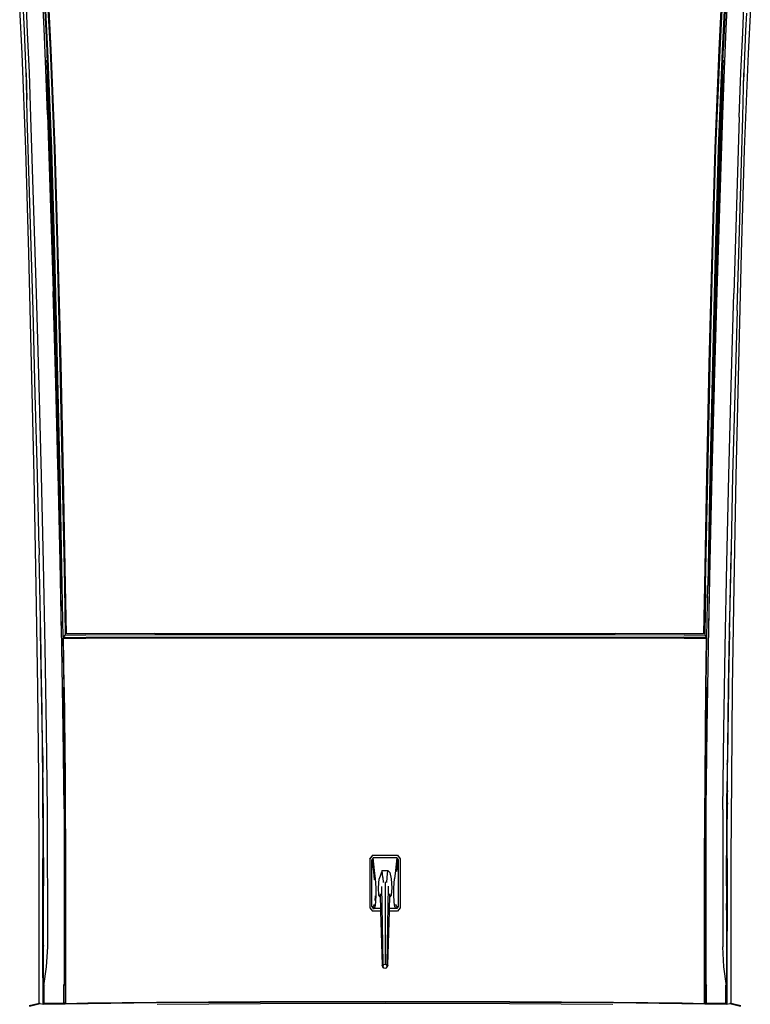
# Model space of a CAD drawing. Units: inches. Extents: x -4737294 to -4736756, y 1716389 to 1717040.
# Tile 9 of 25: x -4737175 to -4737124, y 1716491 to 1716559. Entities that reach past the tile are written whole.
import ezdxf

# ---------------------------------------------------------------- set-up
doc = ezdxf.new("R2010")
doc.units = ezdxf.units.IN
doc.header["$MEASUREMENT"] = 0
doc.layers.add('A-EQPM-VEHI', color=250, linetype='Continuous', lineweight=13)
doc.layers.add('Edges', color=250, linetype='Continuous')

# ---------------------------------------------------------------- blocks, each defined once
blk = doc.blocks.new('Nissan Qashqai pl')
at = {"layer": 'Edges'}
for p, q in [((9.4782, 12.5024), (9.5503, 12.4987)), ((9.5168, 12.4903), (9.4761, 12.4919)), ((9.4862, 12.4961), (9.514, 12.4949)), ((9.514, 12.4949), (9.5811, 12.492)), ((9.5812, 12.4874), (9.5168, 12.4903)), ((9.5503, 12.4987), (9.7029, 12.4926)), ((9.651, 12.4906), (9.5811, 12.492)), ((9.5811, 12.492), (9.594, 12.4914)), ((9.6514, 12.4849), (9.5812, 12.4874)), ((9.9583, 12.4812), (9.651, 12.4906)), ((9.7029, 12.4926), (9.8673, 12.4878)), ((9.8673, 12.4878), (10.0423, 12.4835)), ((11.0581, 12.4738), (11.0614, 12.4872)), ((11.0582, 12.47), (11.0624, 12.4866)), ((9.6514, 12.4849), (9.9312, 12.4761)), ((10.0776, 12.4719), (9.9312, 12.4761)), ((9.9583, 12.4812), (10.091, 12.4775)), ((10.0423, 12.4835), (10.2211, 12.4795)), ((10.2201, 12.4683), (10.0776, 12.4719)), ((10.091, 12.4775), (10.2202, 12.4743)), ((10.2202, 12.4743), (10.2203, 12.4743)), ((10.2203, 12.4743), (10.3353, 12.4717)), ((10.2211, 12.4795), (10.3955, 12.4762)), ((10.3353, 12.4717), (10.4477, 12.4694)), ((10.3353, 12.4717), (10.346, 12.4714)), ((10.346, 12.4714), (10.4477, 12.4694)), ((10.3955, 12.4762), (10.5572, 12.4737)), ((10.5572, 12.4737), (10.7004, 12.4722)), ((10.7004, 12.4722), (10.8279, 12.4715)), ((10.8279, 12.4715), (11.0544, 12.4714)), ((11.0544, 12.4714), (11.0575, 12.4714)), ((11.0575, 12.4714), (11.0581, 12.4738)), ((11.0575, 12.4714), (11.0582, 12.47)), ((11.0592, 12.4653), (11.0582, 12.47)), ((9.4694, 12.4654), (9.5105, 12.4637)), ((9.4706, 12.4561), (9.5443, 12.4522)), ((9.5446, 12.4542), (9.4709, 12.4581)), ((9.472, 12.463), (9.5454, 12.4591)), ((9.472, 12.4614), (9.5454, 12.4576)), ((9.5105, 12.4637), (9.5755, 12.4608)), ((9.5454, 12.4591), (9.5454, 12.4593)), ((9.5695, 12.4589), (9.5454, 12.4591)), ((9.5454, 12.4576), (9.7014, 12.4513)), ((9.5609, 12.4593), (9.5695, 12.4589)), ((9.5786, 12.4588), (9.5695, 12.4589)), ((9.5695, 12.4589), (9.7014, 12.4536)), ((9.5755, 12.4608), (9.6472, 12.4581)), ((9.6206, 12.4581), (9.5786, 12.4588)), ((9.6714, 12.4567), (9.6206, 12.4581)), ((9.6414, 12.458), (9.6407, 12.458)), ((9.6472, 12.4581), (9.9278, 12.4492)), ((9.6549, 12.4576), (9.6558, 12.4574)), ((9.6825, 12.4564), (9.6714, 12.4567)), ((9.6825, 12.4564), (9.6829, 12.4563)), ((9.6943, 12.456), (9.6825, 12.4564)), ((9.6943, 12.4558), (9.6943, 12.456)), ((9.6951, 12.456), (9.6943, 12.456)), ((9.6951, 12.4558), (9.6951, 12.456)), ((9.8565, 12.451), (9.6951, 12.456)), ((10.3586, 12.4651), (10.2201, 12.4683)), ((10.4931, 12.4624), (10.3586, 12.4651)), ((10.4477, 12.4694), (10.4538, 12.4693)), ((10.4538, 12.4693), (10.4681, 12.469)), ((10.4676, 12.4691), (10.4538, 12.4693)), ((10.5566, 12.4677), (10.4676, 12.4691)), ((10.4676, 12.4691), (10.546, 12.4677)), ((10.4681, 12.469), (10.5866, 12.467)), ((10.6237, 12.4603), (10.4931, 12.4624)), ((10.546, 12.4677), (10.546, 12.4678)), ((10.546, 12.4677), (10.5576, 12.4675)), ((10.7, 12.4662), (10.5566, 12.4677)), ((10.5576, 12.4675), (10.6649, 12.4659)), ((10.5866, 12.467), (10.6649, 12.4659)), ((10.7502, 12.4586), (10.6237, 12.4603)), ((10.6649, 12.4659), (10.6786, 12.4658)), ((10.6649, 12.4659), (10.6772, 12.4657)), ((10.6786, 12.4657), (10.6772, 12.4657)), ((10.6786, 12.4658), (10.6786, 12.4662)), ((10.6786, 12.4657), (10.6786, 12.4658)), ((10.6786, 12.4658), (10.6801, 12.4657)), ((10.6786, 12.4657), (10.6801, 12.4657)), ((10.6801, 12.4662), (10.6801, 12.4657)), ((10.6801, 12.4657), (10.6801, 12.4657)), ((10.6801, 12.4657), (10.6811, 12.4657)), ((10.6801, 12.4657), (10.6811, 12.4657)), ((10.6811, 12.4662), (10.6811, 12.4657)), ((10.6811, 12.4657), (10.6811, 12.4657)), ((10.6811, 12.4657), (10.6966, 12.4654)), ((10.6811, 12.4657), (10.6991, 12.4655)), ((10.6811, 12.4657), (10.6991, 12.4655)), ((10.6966, 12.4654), (10.7144, 12.4653)), ((10.6991, 12.4655), (10.7144, 12.4653)), ((10.7201, 12.4661), (10.7, 12.4662)), ((10.7144, 12.4653), (10.7239, 12.4653)), ((10.7201, 12.4661), (10.7306, 12.4653)), ((10.7395, 12.4659), (10.7201, 12.4661)), ((10.7239, 12.4653), (10.7248, 12.4653)), ((10.7306, 12.4653), (10.7248, 12.4653)), ((10.7311, 12.4652), (10.7306, 12.4653)), ((10.7495, 12.4652), (10.7311, 12.4652)), ((10.7311, 12.4652), (10.7502, 12.4651)), ((10.7395, 12.4659), (10.7495, 12.4652)), ((10.7923, 12.4656), (10.7395, 12.4659)), ((10.8179, 12.4648), (10.7495, 12.4652)), ((10.7502, 12.4651), (10.7504, 12.4651)), ((10.7502, 12.4586), (10.968, 12.4585)), ((10.7504, 12.4651), (10.7808, 12.4649)), ((10.7808, 12.4649), (10.8179, 12.4648)), ((10.7923, 12.4652), (10.7923, 12.4656)), ((10.7933, 12.4656), (10.7923, 12.4656)), ((10.7933, 12.4652), (10.7933, 12.4656)), ((10.804, 12.4656), (10.7933, 12.4656)), ((10.804, 12.4653), (10.804, 12.4656)), ((10.8075, 12.4655), (10.804, 12.4656)), ((10.8075, 12.4655), (10.8075, 12.4653)), ((10.811, 12.4655), (10.8075, 12.4655)), ((10.811, 12.4655), (10.811, 12.4653)), ((10.8145, 12.4655), (10.811, 12.4655)), ((10.8145, 12.4653), (10.8145, 12.4655)), ((10.8279, 12.4654), (10.8145, 12.4655)), ((10.8277, 12.4647), (10.8179, 12.4648)), ((10.8711, 12.4646), (10.8277, 12.4647)), ((10.8279, 12.4654), (11.0592, 12.4653)), ((10.8711, 12.4646), (10.8824, 12.4646)), ((10.8824, 12.4646), (10.8825, 12.4646)), ((10.8825, 12.4646), (10.8884, 12.4646)), ((10.8884, 12.4646), (10.8923, 12.4646)), ((10.8923, 12.4646), (10.8996, 12.4646)), ((10.9097, 12.4646), (10.8996, 12.4646)), ((10.9097, 12.4646), (10.9399, 12.4646)), ((10.9399, 12.4646), (10.9491, 12.4645)), ((10.9491, 12.4645), (11.0301, 12.4645)), ((11, 12.4605), (10.968, 12.4585)), ((11.0301, 12.4645), (11, 12.4605)), ((11.0301, 12.4637), (11.0287, 12.4637)), ((11.03, 12.4635), (11.0301, 12.4637)), ((11.0301, 12.4642), (11.0301, 12.4645)), ((11.0574, 12.4637), (11.0301, 12.4637)), ((11.0568, 12.4323), (11.0574, 12.4637)), ((11.0574, 12.4637), (11.0592, 12.4653)), ((11.0585, 12.43), (11.0592, 12.4653)), ((9.5443, 12.4522), (9.701, 12.4459)), ((9.7011, 12.4478), (9.5446, 12.4542)), ((9.701, 12.4459), (9.8673, 12.441)), ((9.8673, 12.443), (9.7011, 12.4478)), ((9.7014, 12.4536), (9.8673, 12.4488)), ((9.7014, 12.4513), (9.8673, 12.4464)), ((9.9794, 12.4475), (9.8565, 12.451)), ((9.8673, 12.4488), (10.0429, 12.4444)), ((9.8673, 12.4464), (10.0429, 12.4421)), ((10.043, 12.4387), (9.8673, 12.443)), ((9.8673, 12.441), (10.0431, 12.4367)), ((9.9278, 12.4492), (10.0747, 12.445)), ((10.0998, 12.4443), (9.9794, 12.4475)), ((10.0429, 12.4444), (10.2216, 12.4404)), ((10.0429, 12.4421), (10.2215, 12.4381)), ((10.2218, 12.4347), (10.043, 12.4387)), ((10.0747, 12.445), (10.078, 12.4449)), ((10.078, 12.4449), (10.2146, 12.4414)), ((10.2146, 12.4414), (10.0998, 12.4443)), ((10.2146, 12.4414), (10.2175, 12.4413)), ((10.2175, 12.4413), (10.3564, 12.4382)), ((10.2216, 12.4404), (10.3947, 12.4371)), ((10.0431, 12.4367), (10.2218, 12.4327)), ((10.2215, 12.4381), (10.3945, 12.4348)), ((10.3947, 12.4314), (10.2218, 12.4347)), ((10.2218, 12.4327), (10.3947, 12.4294)), ((10.3564, 12.4382), (10.4638, 12.436)), ((10.4773, 12.4335), (10.3945, 12.4348)), ((10.3947, 12.4371), (10.4638, 12.436)), ((10.3947, 12.4314), (10.4735, 12.4301)), ((10.3947, 12.4294), (10.4715, 12.4282)), ((10.4638, 12.436), (10.4914, 12.4355)), ((10.4715, 12.4282), (10.4711, 12.3973)), ((10.4731, 12.3973), (10.4735, 12.4301)), ((10.4735, 12.4301), (10.4773, 12.4335)), ((10.4773, 12.4296), (10.4769, 12.3968)), ((10.4773, 12.4335), (10.4773, 12.4296)), ((10.4785, 12.433), (10.4773, 12.4335)), ((10.5561, 12.4323), (10.4773, 12.4335)), ((10.4781, 12.3972), (10.4785, 12.433)), ((10.5563, 12.4318), (10.4785, 12.433)), ((10.4914, 12.4355), (10.6223, 12.4333)), ((10.5561, 12.4323), (10.6996, 12.4308)), ((10.6999, 12.4304), (10.5563, 12.4318)), ((10.6223, 12.4333), (10.7493, 12.4316)), ((10.6996, 12.4308), (10.7722, 12.4304)), ((10.827, 12.4297), (10.6999, 12.4304)), ((10.7493, 12.4316), (11.0294, 12.4315)), ((10.7722, 12.4304), (10.7722, 12.4302)), ((10.7722, 12.4304), (10.7889, 12.4303)), ((10.7889, 12.4302), (10.7889, 12.4303)), ((10.7889, 12.4303), (10.7923, 12.4303)), ((10.7923, 12.4302), (10.7923, 12.4303)), ((10.7923, 12.4303), (10.7933, 12.4303)), ((10.7933, 12.4302), (10.7933, 12.4303)), ((10.7933, 12.4303), (10.8267, 12.4301)), ((10.8267, 12.4301), (11.0585, 12.43)), ((10.9133, 12.4296), (10.827, 12.4297)), ((10.9133, 12.4296), (10.9133, 12.4298)), ((10.9137, 12.4296), (10.9133, 12.4296)), ((10.9137, 12.4296), (10.9138, 12.4298)), ((10.9715, 12.4296), (10.9137, 12.4296)), ((10.9715, 12.4299), (10.9715, 12.4296)), ((11.0579, 12.4296), (10.9715, 12.4296)), ((11.0281, 12.4323), (11.0568, 12.4323)), ((11.0294, 12.4315), (11.0294, 12.4316)), ((11.0295, 12.4341), (11.0295, 12.4343)), ((11.0568, 12.4323), (11.0585, 12.43)), ((11.0572, 12.3942), (11.0579, 12.4296)), ((11.0579, 12.3938), (11.0585, 12.43)), ((11.0579, 12.4296), (11.0585, 12.43)), ((10.4711, 12.3973), (10.4706, 12.2875)), ((10.4726, 12.2875), (10.4731, 12.3973)), ((10.4764, 12.2872), (10.4769, 12.3968)), ((10.4776, 12.2874), (10.4781, 12.3972)), ((11.056, 12.2851), (11.0572, 12.3942)), ((11.0566, 12.2849), (11.0579, 12.3938)), ((10.4706, 11.5566), (10.4706, 12.2875)), ((10.4726, 11.5567), (10.4726, 12.2875)), ((10.4764, 11.5569), (10.4764, 12.2872)), ((10.4776, 11.5567), (10.4776, 12.2874)), ((11.0551, 12.1203), (11.056, 12.2851)), ((11.0557, 12.1202), (11.0566, 12.2849)), ((11.0595, 12.2842), (11.0586, 12.1198)), ((11.0547, 11.9221), (11.0551, 12.1203)), ((11.0554, 11.9221), (11.0557, 12.1202)), ((11.0586, 12.1198), (11.0583, 11.9221)), ((10.8228, 11.9421), (10.8224, 11.9421)), ((10.8228, 11.9421), (10.8283, 11.9461)), ((10.8228, 11.9021), (10.8228, 11.9421)), ((10.827, 11.9408), (10.8301, 11.9431)), ((10.827, 11.9408), (10.827, 11.9033)), ((10.827, 11.9408), (10.8467, 11.9386)), ((10.8279, 11.9461), (10.8283, 11.9461)), ((10.8283, 11.9461), (10.906, 11.9461)), ((10.8483, 11.9406), (10.8301, 11.9431)), ((10.8301, 11.9431), (10.9043, 11.9431)), ((10.8467, 11.9386), (10.8603, 11.9373)), ((10.9035, 11.9403), (10.9008, 11.9391)), ((10.905, 11.9414), (10.9035, 11.9403)), ((10.9043, 11.9431), (10.9074, 11.9408)), ((10.9043, 11.9431), (10.905, 11.9414)), ((10.9074, 11.9393), (10.9057, 11.9384)), ((10.906, 11.9461), (10.9116, 11.9421)), ((10.9074, 11.9408), (10.9074, 11.9393)), ((10.9074, 11.9393), (10.9074, 11.9291)), ((10.9116, 11.9421), (10.9116, 11.929)), ((10.8467, 11.9263), (10.8501, 11.9295)), ((10.8467, 11.9178), (10.8467, 11.9263)), ((10.8579, 11.9255), (10.8467, 11.9263)), ((10.8501, 11.9295), (10.8603, 11.9316)), ((10.8662, 11.925), (10.8579, 11.9255)), ((10.8746, 11.9363), (10.8603, 11.9373)), ((10.8603, 11.9316), (10.8746, 11.9327)), ((10.9946, 11.9254), (10.872, 11.9276)), ((10.8861, 11.9361), (10.8746, 11.9363)), ((10.8746, 11.9327), (10.8861, 11.9319)), ((10.889, 11.9296), (10.884, 11.9298)), ((10.8959, 11.9365), (10.8861, 11.9361)), ((10.8861, 11.9319), (10.889, 11.9296)), ((10.9074, 11.9291), (10.889, 11.9296)), ((10.9021, 11.9372), (10.8959, 11.9365)), ((10.9057, 11.9384), (10.9021, 11.9372)), ((10.9116, 11.929), (10.9074, 11.9291)), ((10.9973, 11.9268), (10.9116, 11.929)), ((10.9969, 11.9247), (10.9946, 11.9254)), ((10.9969, 11.9247), (10.996, 11.9221)), ((10.999, 11.9258), (10.9969, 11.9247)), ((10.9973, 11.9268), (11.0001, 11.9254)), ((10.999, 11.9258), (10.9973, 11.9268)), ((11.0012, 11.9247), (10.999, 11.9258)), ((11.0012, 11.9247), (11.0001, 11.9254)), ((11.002, 11.9221), (11.0012, 11.9247)), ((10.8579, 11.9187), (10.8467, 11.9178)), ((10.8467, 11.9178), (10.8603, 11.9126)), ((10.8579, 11.9187), (10.8662, 11.9191)), ((10.8746, 11.9115), (10.8603, 11.9126)), ((10.8746, 11.9078), (10.8603, 11.9068)), ((10.8647, 11.9221), (10.996, 11.9221)), ((10.8723, 11.9165), (10.9946, 11.9187)), ((10.8861, 11.9122), (10.8746, 11.9115)), ((10.8861, 11.908), (10.8746, 11.9078)), ((10.884, 11.9144), (10.889, 11.9145)), ((10.889, 11.9145), (10.8861, 11.9122)), ((10.8959, 11.9077), (10.8861, 11.908)), ((10.889, 11.9145), (10.9074, 11.915)), ((10.9021, 11.9069), (10.8959, 11.9077)), ((10.9074, 11.915), (10.9116, 11.9151)), ((10.9074, 11.915), (10.9074, 11.9049)), ((10.9116, 11.9151), (10.9973, 11.9173)), ((10.9116, 11.9151), (10.9116, 11.9021)), ((10.9946, 11.9187), (10.9969, 11.9195)), ((10.996, 11.9221), (10.9969, 11.9195)), ((10.9969, 11.9195), (10.999, 11.9184)), ((11.0001, 11.9187), (10.9973, 11.9173)), ((10.9973, 11.9173), (10.999, 11.9184)), ((10.999, 11.9184), (10.9996, 11.9187)), ((10.9996, 11.9187), (11.0012, 11.9195)), ((11.0001, 11.9187), (10.9996, 11.9187)), ((11.0012, 11.9195), (11.0001, 11.9187)), ((11.0012, 11.9195), (11.002, 11.9221)), ((11.0551, 11.7239), (11.0547, 11.9221)), ((11.0557, 11.724), (11.0554, 11.9221)), ((11.0583, 11.9221), (11.0586, 11.7244)), ((10.8224, 11.9021), (10.8228, 11.9021)), ((10.8228, 11.9021), (10.8283, 11.8981)), ((10.8467, 11.9056), (10.827, 11.9033)), ((10.827, 11.9033), (10.8301, 11.9011)), ((10.8283, 11.8981), (10.8279, 11.8981)), ((10.8283, 11.8981), (10.906, 11.8981)), ((10.8301, 11.9011), (10.8483, 11.9036)), ((10.9043, 11.9011), (10.8301, 11.9011)), ((10.8603, 11.9068), (10.8467, 11.9056)), ((10.8483, 11.9036), (10.8619, 11.905)), ((10.8871, 11.9063), (10.8944, 11.906)), ((10.9008, 11.905), (10.9035, 11.9039)), ((10.9057, 11.9058), (10.9021, 11.9069)), ((10.9035, 11.9039), (10.905, 11.9028)), ((10.9043, 11.9011), (10.9074, 11.9033)), ((10.905, 11.9028), (10.9043, 11.9011)), ((10.9074, 11.9049), (10.9057, 11.9058)), ((10.906, 11.8981), (10.9116, 11.9021)), ((10.9074, 11.9033), (10.9074, 11.9049)), ((10.9074, 11.9033), (10.9074, 11.9048)), ((11.056, 11.559), (11.0551, 11.7239)), ((11.0566, 11.5593), (11.0557, 11.724)), ((11.0586, 11.7244), (11.0595, 11.5599)), ((10.4706, 11.5566), (10.4711, 11.4469)), ((10.4731, 11.4469), (10.4726, 11.5567)), ((10.4769, 11.4474), (10.4764, 11.5569)), ((10.4781, 11.4469), (10.4776, 11.5567)), ((11.0572, 11.4499), (11.056, 11.559)), ((11.0579, 11.4504), (11.0566, 11.5593)), ((10.4711, 11.4469), (10.4715, 11.416)), ((10.4735, 11.414), (10.4731, 11.4469)), ((10.4773, 11.4146), (10.4769, 11.4474)), ((10.4785, 11.4111), (10.4781, 11.4469)), ((11.0579, 11.4146), (11.0572, 11.4499)), ((11.0585, 11.4142), (11.0579, 11.4504)), ((10.0431, 11.4075), (9.8673, 11.4031)), ((10.043, 11.4055), (10.2218, 11.4094)), ((10.2218, 11.4114), (10.0431, 11.4075)), ((10.3945, 11.4094), (10.2215, 11.406)), ((10.3947, 11.4148), (10.2218, 11.4114)), ((10.2218, 11.4094), (10.3947, 11.4128)), ((10.4416, 11.4077), (10.3564, 11.406)), ((10.4773, 11.4107), (10.3945, 11.4094)), ((10.4715, 11.416), (10.3947, 11.4148)), ((10.3947, 11.4128), (10.4735, 11.414)), ((10.4416, 11.4078), (10.3947, 11.4071)), ((10.4519, 11.4079), (10.4416, 11.4077)), ((10.4519, 11.4079), (10.4416, 11.4078)), ((10.4416, 11.4077), (10.4416, 11.4078)), ((10.4524, 11.408), (10.4519, 11.4079)), ((10.4519, 11.4079), (10.4519, 11.4079)), ((10.4524, 11.4079), (10.4519, 11.4079)), ((10.4524, 11.4079), (10.4524, 11.408)), ((10.4533, 11.408), (10.4524, 11.408)), ((10.4533, 11.4079), (10.4524, 11.4079)), ((10.4638, 11.4081), (10.4533, 11.4079)), ((10.4638, 11.4081), (10.4533, 11.408)), ((10.4533, 11.4079), (10.4533, 11.408)), ((10.4914, 11.4087), (10.4638, 11.4081)), ((10.4773, 11.4107), (10.4735, 11.414)), ((10.4773, 11.4146), (10.4773, 11.4107)), ((10.4773, 11.4107), (10.5561, 11.4119)), ((10.4773, 11.4107), (10.4785, 11.4111)), ((10.5563, 11.4123), (10.4785, 11.4111)), ((10.6223, 11.4109), (10.4914, 11.4087)), ((10.6996, 11.4134), (10.5561, 11.4119)), ((10.5563, 11.4123), (10.6999, 11.4138)), ((10.7493, 11.4125), (10.6223, 11.4109)), ((10.7722, 11.4138), (10.6996, 11.4134)), ((10.6999, 11.4138), (10.7722, 11.4142)), ((10.7493, 11.4125), (11.0294, 11.4126)), ((10.7722, 11.4142), (10.7889, 11.4143)), ((10.7722, 11.4142), (10.7722, 11.4138)), ((10.7889, 11.4139), (10.7722, 11.4138)), ((10.7889, 11.4139), (10.7889, 11.4143)), ((10.7889, 11.4143), (10.7923, 11.4143)), ((10.7923, 11.4139), (10.7889, 11.4139)), ((10.7923, 11.4139), (10.7923, 11.4143)), ((10.7923, 11.4143), (10.7933, 11.4143)), ((10.7933, 11.4139), (10.7923, 11.4139)), ((10.7933, 11.4143), (10.827, 11.4145)), ((10.7933, 11.4139), (10.7933, 11.4143)), ((10.8267, 11.4141), (10.7933, 11.4139)), ((10.8267, 11.4141), (11.0585, 11.4142)), ((10.827, 11.4145), (11.0579, 11.4146)), ((11.0294, 11.4118), (11.0281, 11.4118)), ((11.0294, 11.4125), (11.0294, 11.4126)), ((11.0295, 11.4116), (11.0294, 11.4118)), ((11.0568, 11.4118), (11.0294, 11.4118)), ((11.0585, 11.4142), (11.0568, 11.4118)), ((11.0574, 11.3804), (11.0568, 11.4118)), ((11.0585, 11.4142), (11.0579, 11.4146)), ((11.0592, 11.3789), (11.0585, 11.4142)), ((9.5443, 11.3919), (9.4706, 11.388)), ((9.701, 11.3983), (9.5443, 11.3919)), ((9.5446, 11.39), (9.7011, 11.3963)), ((9.7014, 11.3929), (9.5454, 11.3866)), ((9.6472, 11.3861), (9.9278, 11.3949)), ((9.6714, 11.3874), (9.8565, 11.3931)), ((9.8673, 11.4031), (9.701, 11.3983)), ((9.7011, 11.3963), (9.8673, 11.4012)), ((9.8673, 11.3977), (9.7014, 11.3929)), ((9.8673, 11.3954), (9.7014, 11.3906)), ((9.8565, 11.3931), (9.9794, 11.3967)), ((9.8673, 11.4012), (10.043, 11.4055)), ((10.0429, 11.4021), (9.8673, 11.3977)), ((10.0429, 11.3998), (9.8673, 11.3954)), ((10.0747, 11.3991), (9.9278, 11.3949)), ((9.9794, 11.3967), (10.0965, 11.3998)), ((10.2215, 11.406), (10.0429, 11.4021)), ((10.2216, 11.4037), (10.0429, 11.3998)), ((10.2043, 11.4025), (10.0747, 11.3991)), ((10.0965, 11.3998), (10.0998, 11.3999)), ((10.0998, 11.3999), (10.2043, 11.4025)), ((10.2175, 11.4028), (10.2043, 11.4025)), ((10.3564, 11.406), (10.2175, 11.4028)), ((10.3947, 11.4071), (10.2216, 11.4037)), ((9.5105, 11.3805), (9.4694, 11.3788)), ((9.4709, 11.3861), (9.5446, 11.39)), ((9.5454, 11.3866), (9.472, 11.3828)), ((9.472, 11.3812), (9.5454, 11.3851)), ((9.5755, 11.3834), (9.5105, 11.3805)), ((9.5454, 11.3851), (9.5695, 11.3853)), ((9.5454, 11.3848), (9.5454, 11.3851)), ((9.5695, 11.3853), (9.5609, 11.3849)), ((9.7014, 11.3906), (9.5695, 11.3853)), ((9.5695, 11.3853), (9.5786, 11.3853)), ((9.6472, 11.3861), (9.5755, 11.3834)), ((9.5786, 11.3853), (9.6206, 11.3861)), ((9.6206, 11.3861), (9.6714, 11.3874)), ((10.2201, 11.3759), (10.3586, 11.3791)), ((10.3586, 11.3791), (10.4931, 11.3817)), ((10.5576, 11.3766), (10.4676, 11.3751)), ((10.5566, 11.3765), (10.4676, 11.3751)), ((10.5866, 11.3772), (10.4681, 11.3752)), ((10.4931, 11.3817), (10.6237, 11.3839)), ((10.5566, 11.3765), (10.7, 11.378)), ((10.6649, 11.3783), (10.5576, 11.3766)), ((10.6649, 11.3783), (10.5866, 11.3772)), ((10.6237, 11.3839), (10.7502, 11.3855)), ((10.6908, 11.3785), (10.6649, 11.3783)), ((10.6649, 11.3783), (10.6772, 11.3784)), ((10.6966, 11.3787), (10.6772, 11.3784)), ((10.6772, 11.3784), (10.6908, 11.3785)), ((10.6991, 11.3786), (10.6908, 11.3785)), ((10.7144, 11.3788), (10.6966, 11.3787)), ((10.6999, 11.3786), (10.6991, 11.3786)), ((10.6999, 11.3786), (10.7808, 11.3793)), ((10.7144, 11.3788), (10.6999, 11.3786)), ((10.7, 11.378), (10.8279, 11.3787)), ((10.7239, 11.3789), (10.7144, 11.3788)), ((10.7248, 11.3789), (10.7239, 11.3789)), ((10.7808, 11.3793), (10.7248, 11.3789)), ((10.7502, 11.3855), (10.968, 11.3857)), ((10.7808, 11.3793), (10.8711, 11.3796)), ((10.9431, 11.3796), (10.8279, 11.3787)), ((10.8279, 11.3787), (11.0552, 11.3789)), ((10.9614, 11.3788), (10.8279, 11.3787)), ((10.896, 11.3796), (10.8711, 11.3796)), ((10.9097, 11.3796), (10.896, 11.3796)), ((10.9431, 11.3796), (10.9097, 11.3796)), ((10.9478, 11.3796), (10.9431, 11.3796)), ((10.9491, 11.3796), (10.9478, 11.3796)), ((10.9668, 11.3796), (10.9491, 11.3796)), ((10.9614, 11.3788), (10.9668, 11.3796)), ((10.9711, 11.3788), (10.9614, 11.3788)), ((10.9668, 11.3796), (10.967, 11.3796)), ((10.9765, 11.3796), (10.967, 11.3796)), ((10.968, 11.3857), (11, 11.3837)), ((10.9765, 11.3796), (10.9711, 11.3788)), ((10.9766, 11.3788), (10.9711, 11.3788)), ((10.9765, 11.3796), (10.9766, 11.3788)), ((10.9825, 11.3796), (10.9765, 11.3796)), ((11.0592, 11.3789), (10.9766, 11.3788)), ((11.0301, 11.3796), (10.9825, 11.3796)), ((11, 11.3837), (11.0301, 11.3796)), ((11.0287, 11.3804), (11.0301, 11.3804)), ((11.0301, 11.3803), (11.0292, 11.3802)), ((11.03, 11.3822), (11.03, 11.3824)), ((11.0301, 11.3803), (11.0301, 11.3804)), ((11.0301, 11.3804), (11.0554, 11.3804)), ((11.0554, 11.3804), (11.0301, 11.3803)), ((11.0301, 11.3796), (11.0301, 11.3803)), ((11.0554, 11.3804), (11.0574, 11.3804)), ((11.0592, 11.3789), (11.0574, 11.3804)), ((11.0582, 11.3742), (11.0592, 11.3789)), ((9.9583, 11.363), (9.651, 11.3536)), ((9.6514, 11.3592), (9.9312, 11.3681)), ((10.0423, 11.3607), (9.8673, 11.3563)), ((9.9312, 11.3681), (10.0776, 11.3722)), ((10.091, 11.3666), (9.9583, 11.363)), ((10.2211, 11.3646), (10.0423, 11.3607)), ((10.0776, 11.3722), (10.2201, 11.3759)), ((10.2191, 11.3699), (10.091, 11.3666)), ((10.2202, 11.3699), (10.2191, 11.3699)), ((10.2202, 11.3699), (10.2203, 11.3699)), ((10.3353, 11.3725), (10.2203, 11.3699)), ((10.3955, 11.368), (10.2211, 11.3646)), ((10.3353, 11.3725), (10.346, 11.3727)), ((10.4477, 11.3747), (10.346, 11.3727)), ((10.5572, 11.3704), (10.3955, 11.368)), ((10.4537, 11.3749), (10.4477, 11.3747)), ((10.4537, 11.3749), (10.4538, 11.3749)), ((10.4681, 11.3752), (10.4538, 11.3749)), ((10.4676, 11.3751), (10.4538, 11.3749)), ((10.4676, 11.3751), (10.4676, 11.3751)), ((10.7004, 11.372), (10.5572, 11.3704)), ((10.8279, 11.3727), (10.7004, 11.372)), ((11.0544, 11.3728), (10.8279, 11.3727)), ((11.0575, 11.3728), (11.0544, 11.3728)), ((11.0582, 11.3742), (11.0575, 11.3728)), ((11.0581, 11.3704), (11.0575, 11.3728)), ((11.0614, 11.3569), (11.0581, 11.3704)), ((11.0624, 11.3576), (11.0582, 11.3742)), ((9.514, 11.3492), (9.4605, 11.3465)), ((9.4761, 11.3522), (9.5168, 11.3539)), ((9.5503, 11.3455), (9.4782, 11.3418)), ((9.5811, 11.3522), (9.514, 11.3492)), ((9.5168, 11.3539), (9.5812, 11.3568)), ((9.7029, 11.3516), (9.5503, 11.3455)), ((9.5811, 11.3522), (9.6231, 11.3531)), ((9.594, 11.3527), (9.5811, 11.3522)), ((9.5812, 11.3568), (9.6514, 11.3592)), ((9.6231, 11.3531), (9.594, 11.3527)), ((9.651, 11.3536), (9.6231, 11.3531)), ((9.8673, 11.3563), (9.7029, 11.3516))]:
    blk.add_line(p, q, dxfattribs=at)
blk = doc.blocks.new('car')
blk.add_blockref('Nissan Qashqai pl', (-9.7433, -11.9151))

msp = doc.modelspace()

# ---------------------------------------------------------------- block references
at = {"layer": 'A-EQPM-VEHI', "xscale": 43.56002006885659, "yscale": 43.56002006885659, "zscale": 43.56002006885659, "rotation": 270}
msp.add_blockref('car', (-4737150.017, 1716548.61), dxfattribs=at)

doc.saveas('drawing.dxf')
